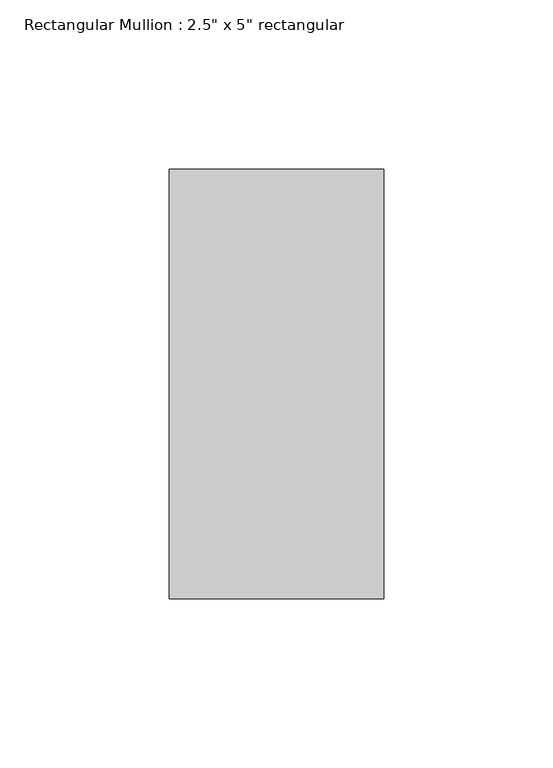
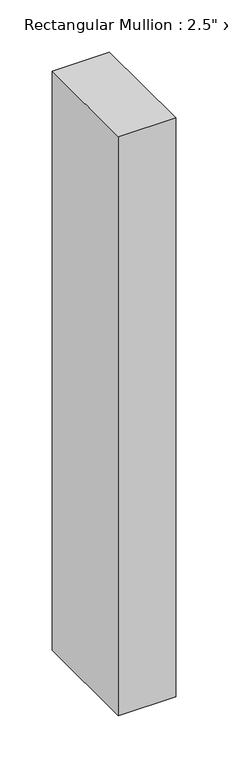
"""IFC4 building model written with IfcOpenShell, lengths in millimetres: member geometry."""

from ifc_helpers import new_model, si_unit, frame, origin, place, context, project, spatial, polyline, outline, extrude, source, transform, mapped, element, save


def member_be967ef6(model_context):
    return source(origin(), model_context, "Body", "SweptSolid", [
        extrude(outline(polyline([(0.0, 63.5), (0.0, -63.5), (-63.5, -63.5), (-63.5, 63.5), (0.0, 63.5)])), frame((0.0, 0.0, -677.9496655), z_axis=(0.0, 0.0, 1.0), x_axis=(1.0, 0.0, 0.0)), (0.0, 0.0, 1.0), 677.9496655),
    ])


if __name__ == "__main__":
    model = new_model("IFC4")
    model_context = context("Model", 3, world=origin())
    ifc_project = project(units=[si_unit("LENGTHUNIT", "METRE", prefix="MILLI")], contexts=[model_context])
    site = spatial("IfcSite", under=ifc_project)
    building = spatial("IfcBuilding", under=site)
    placement = place(None, origin())
    member_shape = member_be967ef6(model_context)
    element("IfcMember", 1, ObjectType="Rectangular Mullion : 2.5\" x 5\" rectangular", at=placement, inside=building, context=model_context, shape_type="MappedRepresentation", body=[
        mapped(member_shape, transform((0.0, 0.0, 0.0), x_axis=(1.0, 0.0, 0.0), y_axis=(0.0, 1.0, 0.0), z_axis=(0.0, 0.0, 1.0))),
    ])
    save(model, "model.ifc")

# Revit data of these elements
# Type "Rectangular Mullion : 2.5\" x 5\" rectangular"
#   built-in parameter 1007304 = 0.416667 (stored number, unit not read)
#   built-in parameter 1007301 = 0.104167 (stored number, unit not read)
#   built-in parameter 1007300 = 0.104167 (stored number, unit not read)
# Element 1 (IfcMember, "Rectangular Mullion : 2.5\" x 5\" rectangular")
#   Materials on its faces: "Aluminum"
# Materials
#   "Aluminum": class "Metal", colour RGB 247 247 247, transparency 0, Description = "Aluminum 6061", Cost = 0
